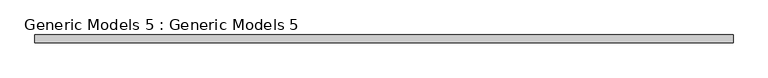
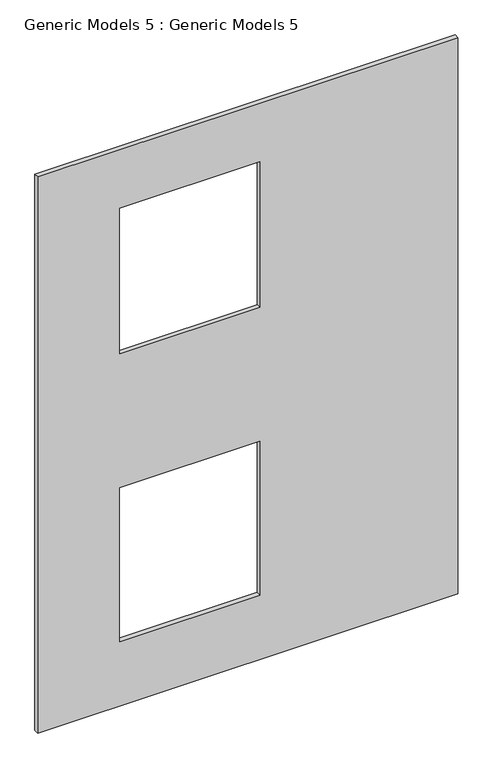
"""IFC4 building model written with IfcOpenShell, lengths in millimetres: proxy geometry, Generic Models 5 : Generic Models 5."""

from ifc_helpers import new_model, si_unit, frame, origin, place, context, project, spatial, polyline, outline, extrude, source, transform, mapped, element, save


def generic_models_5_generic_models_5_fcb812c2(model_context):
    return source(origin(), model_context, "Body", "SweptSolid", [
        extrude(outline(polyline([(6400.8, -12187.5503587), (0.0, -12187.5503587), (0.0, -7615.5503587), (6400.8, -7615.5503587), (6400.8, -12187.5503587)]), holes=[polyline([(5725.9797172, -11292.2003587), (5725.9797172, -9768.2003587), (4050.5645472, -9768.2003587), (4050.5645472, -11292.2003587), (5725.9797172, -11292.2003587)]), polyline([(2511.49538, -9768.2003587), (739.995359, -9768.2003587), (739.995359, -11292.2003587), (2511.49538, -11292.2003587), (2511.49538, -9768.2003587)])]), frame((0.0, -13924.1526331, 0.0), z_axis=(0.0, 1.0, 0.0), x_axis=(0.0, 0.0, 1.0)), (0.0, 0.0, 1.0), 50.8),
    ])


if __name__ == "__main__":
    model = new_model("IFC4")
    model_context = context("Model", 3, world=origin())
    ifc_project = project(units=[si_unit("LENGTHUNIT", "METRE", prefix="MILLI")], contexts=[model_context])
    site = spatial("IfcSite", under=ifc_project)
    building = spatial("IfcBuilding", under=site)
    placement = place(None, origin())
    generic_models_5_generic_models_5_shape = generic_models_5_generic_models_5_fcb812c2(model_context)
    element("IfcBuildingElementProxy", 1, Name="Generic Models 5 : Generic Models 5", ObjectType="Generic Models 5 : Generic Models 5", at=placement, inside=building, context=model_context, shape_type="MappedRepresentation", body=[
        mapped(generic_models_5_generic_models_5_shape, transform((0.0, 0.0, 0.0), x_axis=(1.0, 0.0, 0.0), y_axis=(0.0, 1.0, 0.0), z_axis=(0.0, 0.0, 1.0))),
    ])
    save(model, "model.ifc")
